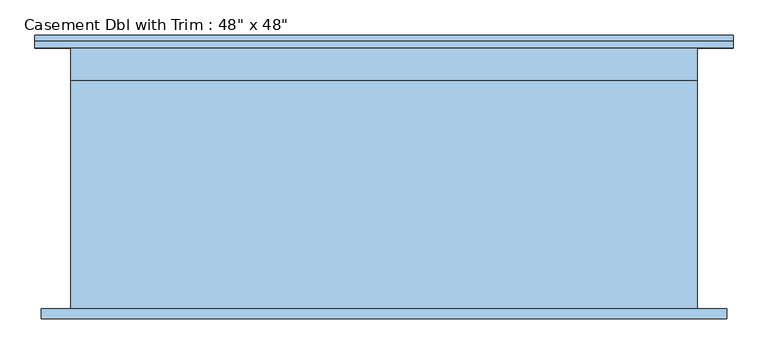
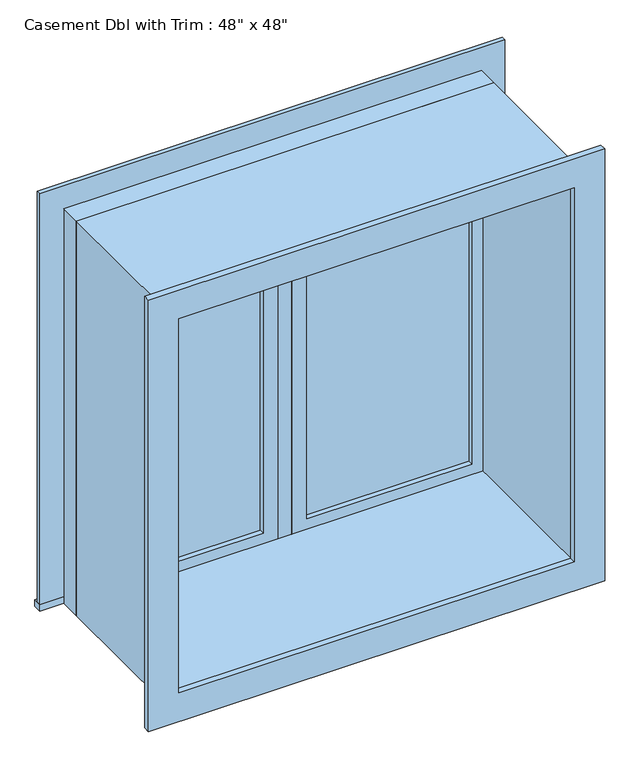
"""IFC4 building model written with IfcOpenShell, lengths in millimetres: window geometry."""

from ifc_helpers import new_model, si_unit, frame, origin, place, context, project, spatial, polyline, outline, extrude, source, transform, mapped, element, save


def window_adfa5946(model_context):
    return source(origin(), model_context, "Body", "SweptSolid", [
        extrude(outline(polyline([(63.5, 238.125), (546.1, 238.125), (546.1, 225.425), (63.5, 225.425), (63.5, 238.125)])), frame((0.0, 0.0, 977.9), z_axis=(0.0, 0.0, 1.0), x_axis=(1.0, 0.0, 0.0)), (0.0, 0.0, 1.0), 1092.2),
        extrude(outline(polyline([(2114.55, 19.05), (933.45, 19.05), (933.45, 590.55), (2114.55, 590.55), (2114.55, 19.05)]), holes=[polyline([(2070.1, 63.5), (2070.1, 546.1), (977.9, 546.1), (977.9, 63.5), (2070.1, 63.5)])]), frame((0.0, 209.55, 0.0), z_axis=(0.0, 1.0, 0.0), x_axis=(0.0, 0.0, 1.0)), (0.0, 0.0, 1.0), 44.45),
        extrude(outline(polyline([(19.05, 209.55), (-19.05, 209.55), (-19.05, 273.05), (19.05, 273.05), (19.05, 209.55)])), frame((0.0, 0.0, 933.45), z_axis=(0.0, 0.0, 1.0), x_axis=(1.0, 0.0, 0.0)), (0.0, 0.0, 1.0), 1181.1),
        extrude(outline(polyline([(-679.45, 298.45), (679.45, 298.45), (679.45, 273.05), (-679.45, 273.05), (-679.45, 298.45)])), frame((0.0, 0.0, 914.4), z_axis=(0.0, 0.0, 1.0), x_axis=(1.0, 0.0, 0.0)), (0.0, 0.0, 1.0), 19.05),
        extrude(outline(polyline([(2114.55, -590.55), (2114.55, 590.55), (933.45, 590.55), (933.45, 679.45), (2203.45, 679.45), (2203.45, -679.45), (933.45, -679.45), (933.45, -590.55), (2114.55, -590.55)])), frame((0.0, 273.05, 0.0), z_axis=(0.0, 1.0, 0.0), x_axis=(0.0, 0.0, 1.0)), (0.0, 0.0, 1.0), 12.7),
        extrude(outline(polyline([(2190.75, 666.75), (2190.75, -666.75), (857.25, -666.75), (857.25, 666.75), (2190.75, 666.75)]), holes=[polyline([(2101.85, 577.85), (946.15, 577.85), (946.15, -577.85), (2101.85, -577.85), (2101.85, 577.85)])]), frame((0.0, -254.0, 0.0), z_axis=(0.0, 1.0, 0.0), x_axis=(0.0, 0.0, 1.0)), (0.0, 0.0, 1.0), 19.05),
        extrude(outline(polyline([(-63.5, 225.425), (-546.1, 225.425), (-546.1, 238.125), (-63.5, 238.125), (-63.5, 225.425)])), frame((0.0, 0.0, 977.9), z_axis=(0.0, 0.0, 1.0), x_axis=(1.0, 0.0, 0.0)), (0.0, 0.0, 1.0), 1092.2),
        extrude(outline(polyline([(2114.55, -590.55), (933.45, -590.55), (933.45, -19.05), (2114.55, -19.05), (2114.55, -590.55)]), holes=[polyline([(2070.1, -546.1), (2070.1, -63.5), (977.9, -63.5), (977.9, -546.1), (2070.1, -546.1)])]), frame((0.0, 209.55, 0.0), z_axis=(0.0, 1.0, 0.0), x_axis=(0.0, 0.0, 1.0)), (0.0, 0.0, 1.0), 44.45),
        extrude(outline(polyline([(2133.6, -609.6), (914.4, -609.6), (914.4, 609.6), (2133.6, 609.6), (2133.6, -609.6)]), holes=[polyline([(2101.85, -577.85), (2101.85, 577.85), (946.15, 577.85), (946.15, -577.85), (2101.85, -577.85)])]), frame((0.0, -234.95, 0.0), z_axis=(0.0, 1.0, 0.0), x_axis=(0.0, 0.0, 1.0)), (0.0, 0.0, 1.0), 444.5),
        extrude(outline(polyline([(2133.6, 609.6), (2133.6, -609.6), (914.4, -609.6), (914.4, 609.6), (2133.6, 609.6)]), holes=[polyline([(2114.55, 590.55), (933.45, 590.55), (933.45, -590.55), (2114.55, -590.55), (2114.55, 590.55)])]), frame((0.0, 209.55, 0.0), z_axis=(0.0, 1.0, 0.0), x_axis=(0.0, 0.0, 1.0)), (0.0, 0.0, 1.0), 63.5),
    ])


if __name__ == "__main__":
    model = new_model("IFC4")
    model_context = context("Model", 3, world=origin())
    ifc_project = project(units=[si_unit("LENGTHUNIT", "METRE", prefix="MILLI")], contexts=[model_context])
    site = spatial("IfcSite", under=ifc_project)
    building = spatial("IfcBuilding", under=site)
    placement = place(None, origin())
    window_shape = window_adfa5946(model_context)
    element("IfcWindow", 1, ObjectType="Casement Dbl with Trim : 48\" x 48\"", at=placement, inside=building, context=model_context, shape_type="MappedRepresentation", body=[
        mapped(window_shape, transform((0.0, 0.0, 0.0), x_axis=(1.0, 0.0, 0.0), y_axis=(0.0, 1.0, 0.0), z_axis=(0.0, 0.0, 1.0))),
    ])
    save(model, "model.ifc")

# Revit data of these elements
# Type "Casement Dbl with Trim : 48\" x 48\""
#   Type Mark = "10"
#   Construction Type Id = "GSP4R"
#   Assembly Code = "B2020100"
#   Analytic Construction = "1/8 in Pilkington single glazing"
#   Visual Light Transmittance = 0.9
#   Solar Heat Gain Coefficient = 0.78
#   Heat Transfer Coefficient (U) = 0.6496 BTU/(h·ft²·°F)
#   Height = 4' - 0"
#   Default Sill Height = 3' - 0"
#   Trim Projection - Ext. = 0' - 0 1/2"
#   Trim Projection - Int. = 0' - 0 3/4"
#   Trim Width - Exterior = 0' - 3 1/2"
#   Trim Width - Interior = 0' - 3 1/2"
#   Width = 4' - 0"
#   Window Inset = 0' - 0 3/4"
#   Define Thermal Properties by = 1
#   Glass Pane Material = Glass
#   Sash Material = Roofing, EPDM Membrane
#   Trim Exterior Material = Roofing, EPDM Membrane
#   Trim Interior Material = Trim
#   Wall Closure = (empty or 0)
# Element 1 (IfcWindow, "Casement Dbl with Trim : 48\" x 48\"")
#   Materials on its faces: "Roofing, EPDM Membrane", "Glass", "Trim"
# Materials
#   "Glass": class "Glass", colour RGB 0 128 192, transparency 0.75, Description = "Soda Lime Glass", Cost = 0
#   "Roofing, EPDM Membrane": class "Generic", colour RGB 127 127 127, transparency 0, Description = "EPDM roof membrane", Cost = 0
#   "Trim": class "Wood", colour RGB 224 178 126, transparency 0
